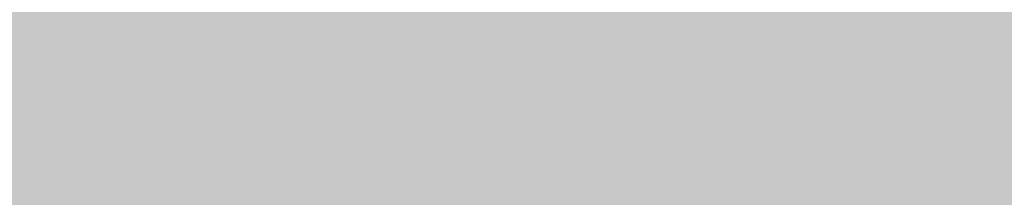
# Model space of a CAD drawing. Units: feet. Extents: x 3168 to 4724, y 827 to 1477.
# Tile 194 of 256: x 3316.07 to 3333.46, y 1093.65 to 1096.78. Entities that reach past the tile are written whole.
import ezdxf

# ---------------------------------------------------------------- set-up
doc = ezdxf.new("R2010")
doc.units = ezdxf.units.FT
doc.layers.add('A-ELEV-PATT', color=8, linetype='Continuous', lineweight=13)

msp = doc.modelspace()

# ---------------------------------------------------------------- hatches: boundary and pattern name
at = {"layer": 'A-ELEV-PATT'}
h = msp.add_hatch(color=256, dxfattribs=at)
h.dxf.hatch_style = 1
edge = h.paths.add_edge_path()
edge.add_ellipse((3552.906, 979.22), major_axis=(36.745, 0), ratio=0.484848, start_angle=0, end_angle=360)
edge = h.paths.add_edge_path()
edge.add_ellipse((3559.892, 929.252), major_axis=(36.745, 0), ratio=0.484848, start_angle=0, end_angle=360)
edge = h.paths.add_edge_path()
edge.add_line((3299.317, 1198.606), (3479.917, 1198.606))
edge.add_line((3479.917, 1198.606), (3479.917, 1209.869))
edge.add_spline(control_points=[(3479.917, 1209.869), (3464.301, 1209.869), (3448.686, 1209.869), (3410.949, 1209.869), (3388.828, 1209.869), (3355.647, 1209.869), (3344.586, 1209.869), (3327.996, 1209.869), (3322.466, 1209.869), (3314.17, 1209.869), (3311.405, 1209.869), (3307.257, 1209.869), (3305.875, 1209.869), (3303.801, 1209.869), (3303.11, 1209.869), (3302.073, 1209.869), (3301.727, 1209.869), (3301.209, 1209.869), (3301.036, 1209.869), (3300.777, 1209.869), (3300.69, 1209.869), (3300.561, 1209.869), (3300.517, 1209.869), (3300.453, 1209.869), (3300.431, 1209.869), (3300.399, 1209.869), (3300.388, 1209.869), (3300.366, 1209.869), (3300.346, 1209.869), (3300.346, 1209.869), (3300.346, 1209.869), (3300.343, 1209.869), (3300.341, 1209.869), (3300.338, 1209.869), (3300.337, 1209.869), (3300.334, 1209.869), (3300.332, 1209.869), (3300.326, 1209.869), (3300.321, 1209.869), (3300.311, 1209.869), (3300.306, 1209.869), (3300.291, 1209.869), (3300.28, 1209.869), (3300.232, 1209.869), (3300.195, 1209.869), (3299.951, 1209.871), (3299.745, 1209.874), (3299.437, 1209.883), (3299.334, 1209.887), (3299.181, 1209.893), (3299.13, 1209.895), (3298.652, 1209.917), (3298.229, 1209.946), (3297.602, 1210.002), (3297.393, 1210.023), (3297.083, 1210.058), (3296.979, 1210.07), (3296.293, 1210.155), (3295.718, 1210.243), (3294.869, 1210.399), (3294.588, 1210.454), (3294.169, 1210.543), (3294.03, 1210.574), (3291.707, 1211.101), (3289.654, 1211.813), (3285.776, 1213.564), (3283.951, 1214.603), (3280.512, 1216.98), (3278.897, 1218.318), (3276.38, 1220.829), (3275.416, 1221.918), (3274.039, 1223.708), (3273.581, 1224.35), (3273.143, 1225.016)], knot_values=[39.119033, 39.119033, 39.119033, 39.119033, 39.286353, 39.286353, 39.523379, 39.523379, 39.641892, 39.641892, 39.701148, 39.701148, 39.730777, 39.730777, 39.745591, 39.745591, 39.752998, 39.752998, 39.756701, 39.756701, 39.758553, 39.758553, 39.759479, 39.759479, 39.759942, 39.759942, 39.760173, 39.760173, 39.760289, 39.760289, 39.760405, 39.760405, 39.760463, 39.760463, 39.763389, 39.763389, 39.764851, 39.764851, 39.767304, 39.767304, 39.773825, 39.773825, 39.78057, 39.78057, 39.79477, 39.79477, 39.845194, 39.845194, 40.126715, 40.126715, 40.267476, 40.267476, 40.337856, 40.337856, 40.927023, 40.927023, 41.221606, 41.221606, 41.368898, 41.368898, 42.202622, 42.202622, 42.619485, 42.619485, 42.827916, 42.827916, 46.118323, 46.118323, 49.408731, 49.408731, 52.699139, 52.699139, 54.927489, 54.927489, 56.104228, 56.104228, 56.104228, 56.104228], weights=[1, 1, 1, 1, 1, 1, 1, 1, 1, 1, 1, 1, 1, 1, 1, 1, 1, 1, 1, 1, 1, 1, 1, 1, 1, 1, 1, 1, 1, 1, 1, 1, 1, 1, 1, 1, 1, 1, 1, 1, 1, 1, 1, 1, 1, 1, 1, 1, 1, 1, 1, 1, 1, 1, 1, 1, 1, 1, 1, 1, 1, 1, 1, 1, 1, 1, 1, 1, 1, 1, 1, 1, 1, 1], degree=3, periodic=0)
edge.add_line((3273.143, 1225.016), (3273.143, 1099.016))
edge.add_line((3273.143, 1099.016), (3299.317, 1099.016))
edge.add_line((3299.317, 1099.016), (3299.317, 1198.606))
edge = h.paths.add_edge_path()
edge.add_line((3304.758, 1324.158), (3479.917, 1324.158))
edge.add_line((3479.917, 1324.158), (3479.917, 1335.715))
edge.add_line((3479.917, 1335.715), (3269.162, 1335.715))
edge.add_spline(control_points=[(3269.162, 1335.715), (3264.024, 1335.715), (3258.364, 1328.958), (3259.264, 1323.9)], knot_values=[0, 0, 0, 0, 15.412191, 15.412191, 15.412191, 15.412191], degree=3, periodic=0)
edge.add_line((3259.264, 1323.9), (3265.517, 1288.769))
edge.add_line((3265.517, 1288.769), (3275.265, 1261.546))
edge.add_line((3275.265, 1261.546), (3304.758, 1261.546))
edge.add_line((3304.758, 1261.546), (3304.758, 1324.158))
h = msp.add_hatch(color=256, dxfattribs=at)
h.dxf.hatch_style = 1
h.paths.add_polyline_path([(3384.525, 1099.016), (3335.029, 1099.016), (3299.317, 1099.016), (3273.143, 1099.016), (3217.565, 1099.016), (3168.069, 827.116), (3335.029, 827.116)])

doc.saveas('drawing.dxf')
